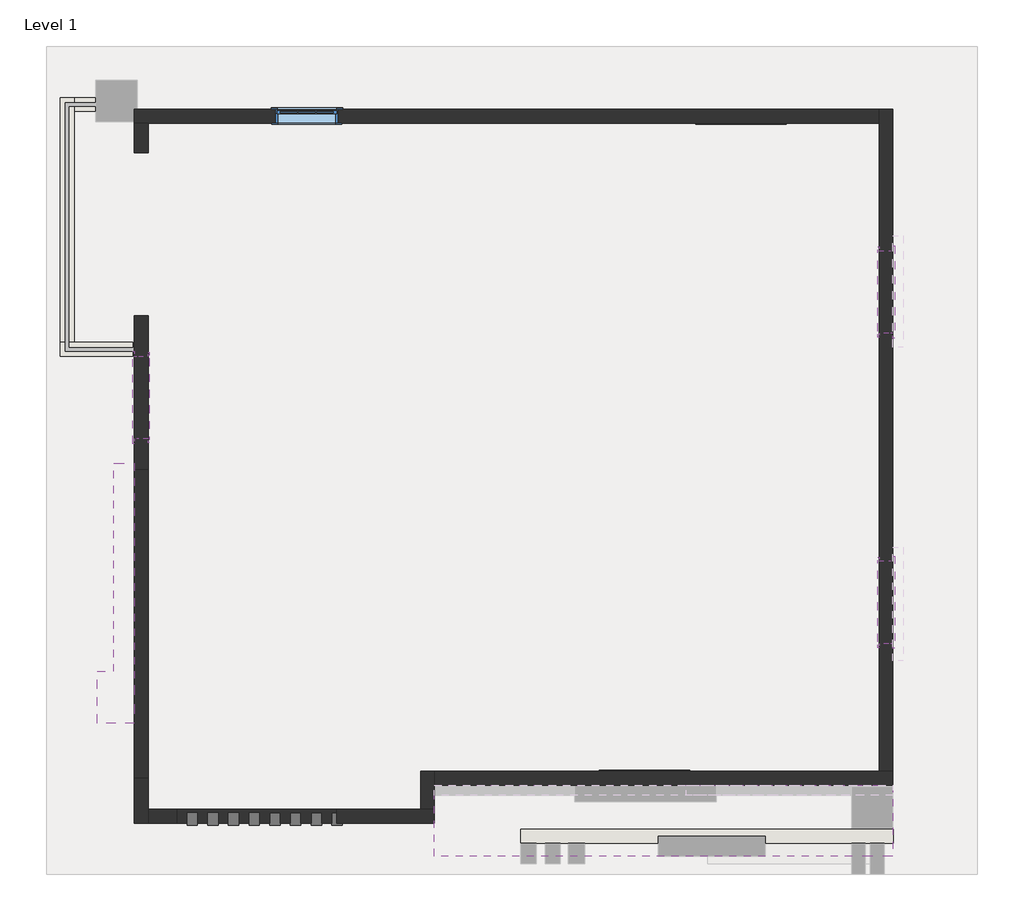
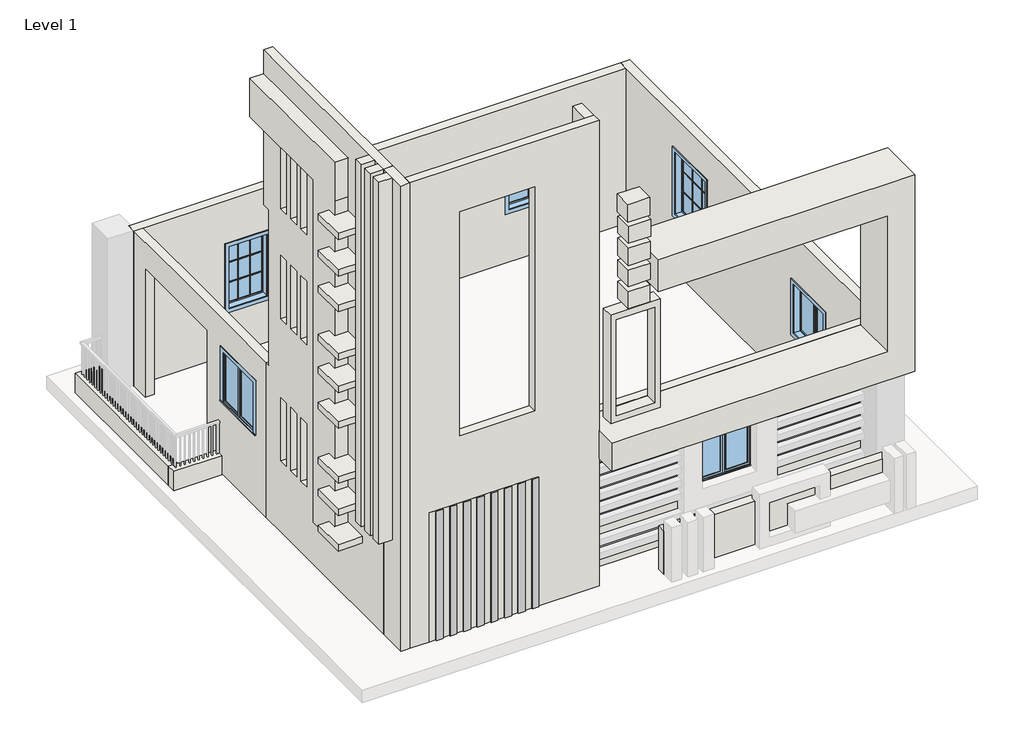
# One storey, part 1 of 2: 15 walls, 8 proxies, 6 windows.
"""IFC4 building model written with IfcOpenShell, lengths in millimetres."""

from ifc_helpers import new_model, si_unit, origin, origin_with_axes, place, context, project, spatial, polyline, outline, extrude, faceted_brep, transform, mapped, element, save
from components import walls_1_walls_1_66469eba, walls_2_walls_2_6b9d7f67, window_58e1470a, window_26ecbd3e, window_0862ab64

model = new_model("IFC4")

# Units and contexts
model_context = context("Model", 3, world=origin())
ifc_project = project(units=[si_unit("LENGTHUNIT", "METRE", prefix="MILLI")], contexts=[model_context])

# Site, building, storey
site = spatial("IfcSite", under=ifc_project)
building = spatial("IfcBuilding", under=site)
storey = spatial("IfcBuildingStorey", under=building, Name="Level 1", Elevation=0.0)

# Proxies
placement = place(None, origin())
element("IfcBuildingElementProxy", 1, Name="Reveal", ObjectType="Reveal", at=placement, inside=storey, context=model_context, shape_type="SweptSolid", body=[
    extrude(outline(polyline([(-11010.4950134, -2653.806099), (-11010.4950134, -2470.926099), (-10858.0950134, -2470.926099), (-10858.0950134, -2653.806099), (-11010.4950134, -2653.806099)])), origin_with_axes(), (0.0, 0.0, 1.0), 3049.7998229),
])
element("IfcBuildingElementProxy", 2, Name="Reveal", ObjectType="Reveal", at=placement, inside=storey, context=model_context, shape_type="SweptSolid", body=[
    extrude(outline(polyline([(-10705.6950134, -2653.806099), (-10705.6950134, -2470.926099), (-10553.2950134, -2470.926099), (-10553.2950134, -2653.806099), (-10705.6950134, -2653.806099)])), origin_with_axes(), (0.0, 0.0, 1.0), 3049.7998229),
])
element("IfcBuildingElementProxy", 3, Name="Reveal", ObjectType="Reveal", at=placement, inside=storey, context=model_context, shape_type="SweptSolid", body=[
    extrude(outline(polyline([(-10400.8950134, -2653.806099), (-10400.8950134, -2470.926099), (-10248.4950134, -2470.926099), (-10248.4950134, -2653.806099), (-10400.8950134, -2653.806099)])), origin_with_axes(), (0.0, 0.0, 1.0), 3049.7998229),
])
element("IfcBuildingElementProxy", 4, Name="Reveal", ObjectType="Reveal", at=placement, inside=storey, context=model_context, shape_type="SweptSolid", body=[
    extrude(outline(polyline([(-10096.0950134, -2653.806099), (-10096.0950134, -2470.926099), (-9943.6950134, -2470.926099), (-9943.6950134, -2653.806099), (-10096.0950134, -2653.806099)])), origin_with_axes(), (0.0, 0.0, 1.0), 3049.7998229),
])
element("IfcBuildingElementProxy", 5, Name="Reveal", ObjectType="Reveal", at=placement, inside=storey, context=model_context, shape_type="SweptSolid", body=[
    extrude(outline(polyline([(-9791.2950134, -2653.806099), (-9791.2950134, -2470.926099), (-9638.8950134, -2470.926099), (-9638.8950134, -2653.806099), (-9791.2950134, -2653.806099)])), origin_with_axes(), (0.0, 0.0, 1.0), 3049.7998229),
])
element("IfcBuildingElementProxy", 6, Name="Reveal", ObjectType="Reveal", at=placement, inside=storey, context=model_context, shape_type="SweptSolid", body=[
    extrude(outline(polyline([(-9486.4950134, -2653.806099), (-9486.4950134, -2470.926099), (-9334.0950134, -2470.926099), (-9334.0950134, -2653.806099), (-9486.4950134, -2653.806099)])), origin_with_axes(), (0.0, 0.0, 1.0), 3049.7998229),
])
element("IfcBuildingElementProxy", 7, Name="Reveal", ObjectType="Reveal", at=placement, inside=storey, context=model_context, shape_type="SweptSolid", body=[
    extrude(outline(polyline([(-9181.6950134, -2653.806099), (-9181.6950134, -2470.926099), (-9029.2950134, -2470.926099), (-9029.2950134, -2653.806099), (-9181.6950134, -2653.806099)])), origin_with_axes(), (0.0, 0.0, 1.0), 3049.7998229),
])
element("IfcBuildingElementProxy", 8, Name="Reveal", ObjectType="Reveal", at=placement, inside=storey, context=model_context, shape_type="SweptSolid", body=[
    extrude(outline(polyline([(-8876.8950134, -2653.806099), (-8876.8950134, -2470.926099), (-8724.4950134, -2470.926099), (-8724.4950134, -2653.806099), (-8876.8950134, -2653.806099)])), origin_with_axes(), (0.0, 0.0, 1.0), 3049.7998229),
])

# Walls
element("IfcWall", 9, ObjectType="Generic - 8\"", at=placement, inside=storey, context=model_context, shape_type="Brep", body=[
    faceted_brep([(-11786.2932708, 7689.073901, 0.0), (-11583.0932708, 7689.073901, 0.0), (-813.4932708, 7689.073901, 0.0), (-813.4932708, 7689.073901, 3657.6), (-11583.0932708, 7689.073901, 3657.6), (-11786.2932708, 7689.073901, 3657.6), (-8789.0932708, 7689.073901, 2590.7953104), (-8789.0932708, 7689.073901, 1066.7953104), (-9703.4932708, 7689.073901, 1066.7953104), (-9703.4932708, 7689.073901, 2590.7953104), (-2235.8932708, 7689.073901, 2428.7388642), (-2235.8932708, 7689.073901, 1209.5388642), (-3455.0932708, 7689.073901, 1209.5388642), (-3455.0932708, 7689.073901, 2428.7388642), (-11786.2932708, 7892.273901, 0.0), (-11786.2932708, 7892.273901, 3657.6), (-11742.7083357, 7892.273901, 3657.6), (-813.4932708, 7892.273901, 3657.6), (-813.4932708, 7892.273901, 0.0), (-11742.7083357, 7892.273901, 0.0), (-8789.0932708, 7892.273901, 2590.7953104), (-9703.4932708, 7892.273901, 2590.7953104), (-9703.4932708, 7892.273901, 1066.7953104), (-8789.0932708, 7892.273901, 1066.7953104), (-2235.8932708, 7892.273901, 2428.7388642), (-3455.0932708, 7892.273901, 2428.7388642), (-3455.0932708, 7892.273901, 1209.5388642), (-2235.8932708, 7892.273901, 1209.5388642), (-11786.2932708, 7709.3483652, 0.0), (-11786.2932708, 7709.3483652, 3657.6)], [[[0, 1, 2, 3, 4, 5], [6, 7, 8, 9], [10, 11, 12, 13]], [[14, 15, 16, 17, 18, 19], [20, 21, 22, 23], [24, 25, 26, 27]], [[2, 1, 0, 28, 14, 19, 18]], [[5, 4, 3, 17, 16, 15, 29]], [[0, 5, 29, 15, 14, 28]], [[3, 2, 18, 17]], [[7, 6, 20, 23]], [[8, 7, 23, 22]], [[9, 8, 22, 21]], [[6, 9, 21, 20]], [[11, 10, 24, 27]], [[12, 11, 27, 26]], [[13, 12, 26, 25]], [[10, 13, 25, 24]]]),
])
element("IfcWall", 10, ObjectType="Generic - 8\"", at=placement, inside=storey, context=model_context, shape_type="Brep", body=[
    faceted_brep([(-11583.0932708, 2578.5483652, 3657.6), (-11583.0932708, 2578.5483652, 0.0), (-11583.0932708, 4851.2528272, 0.0), (-11583.0932708, 4851.2528272, 3042.8682475), (-11583.0932708, 7251.0434239, 3042.8682475), (-11583.0932708, 7251.0434239, 0.0), (-11583.0932708, 7689.073901, 0.0), (-11583.0932708, 7689.073901, 3657.6), (-11583.0932708, 5905.4772304, 3657.6), (-11583.0932708, 4533.8772304, 3657.6), (-11583.0932708, 4254.9483652, 2926.4797977), (-11583.0932708, 4254.9483652, 1707.2797977), (-11583.0932708, 3035.7483652, 1707.2797977), (-11583.0932708, 3035.7483652, 2926.4797977), (-11786.2932708, 2578.5483652, 0.0), (-11786.2932708, 2578.5483652, 3657.6), (-11786.2932708, 4533.8772304, 3657.6), (-11786.2932708, 5905.4772304, 3657.6), (-11786.2932708, 7689.073901, 3657.6), (-11786.2932708, 7689.073901, 0.0), (-11786.2932708, 7251.0434239, 0.0), (-11786.2932708, 7251.0434239, 3042.8682475), (-11786.2932708, 4851.2528272, 3042.8682475), (-11786.2932708, 4851.2528272, 0.0), (-11786.2932708, 4254.9483652, 2926.4797977), (-11786.2932708, 3035.7483652, 2926.4797977), (-11786.2932708, 3035.7483652, 1707.2797977), (-11786.2932708, 4254.9483652, 1707.2797977)], [[[0, 1, 2, 3, 4, 5, 6, 7, 8, 9], [10, 11, 12, 13]], [[14, 15, 16, 17, 18, 19, 20, 21, 22, 23], [24, 25, 26, 27]], [[7, 6, 19, 18]], [[11, 10, 24, 27]], [[12, 11, 27, 26]], [[13, 12, 26, 25]], [[10, 13, 25, 24]], [[0, 9, 8, 7, 18, 17, 16, 15]], [[0, 15, 14, 1]], [[2, 1, 14, 23]], [[3, 2, 23, 22]], [[4, 3, 22, 21]], [[5, 4, 21, 20]], [[6, 5, 20, 19]]]),
])
element("IfcWall", 11, ObjectType="Generic - 8\"", at=placement, inside=storey, context=model_context, shape_type="Brep", body=[
    faceted_brep([(-610.2932708, -1861.326099, 0.0), (-813.4932708, -1861.326099, 0.0), (-7366.6932708, -1861.326099, 0.0), (-7366.6932708, -1861.326099, 3657.6), (-813.4932708, -1861.326099, 3657.6), (-610.2932708, -1861.326099, 3657.6), (-4877.4932708, -1861.326099, 2439.58165), (-4877.4932708, -1861.326099, 1220.38165), (-3658.2932708, -1861.326099, 1220.38165), (-3658.2932708, -1861.326099, 2439.58165), (-610.2932708, -2064.526099, 0.0), (-610.2932708, -2064.526099, 3657.6), (-7366.6932708, -2064.526099, 3657.6), (-7366.6932708, -2064.526099, 0.0), (-4877.4932708, -2064.526099, 2439.58165), (-3658.2932708, -2064.526099, 2439.58165), (-3658.2932708, -2064.526099, 1220.38165), (-4877.4932708, -2064.526099, 1220.38165)], [[[0, 1, 2, 3, 4, 5], [6, 7, 8, 9]], [[10, 11, 12, 13], [14, 15, 16, 17]], [[2, 1, 0, 10, 13]], [[5, 4, 3, 12, 11]], [[0, 5, 11, 10]], [[3, 2, 13, 12]], [[7, 6, 14, 17]], [[8, 7, 17, 16]], [[9, 8, 16, 15]], [[6, 9, 15, 14]]]),
])
element("IfcWall", 12, ObjectType="Generic - 8\"", at=placement, inside=storey, context=model_context, shape_type="Brep", body=[
    faceted_brep([(-813.4932708, 7892.273901, 0.0), (-813.4932708, 7689.073901, 0.0), (-813.4932708, -1861.326099, 0.0), (-813.4932708, -1861.326099, 3657.6), (-813.4932708, 7689.073901, 3657.6), (-813.4932708, 7892.273901, 3657.6), (-813.4932708, 4590.273901, 2873.0721634), (-813.4932708, 4590.273901, 1349.0721634), (-813.4932708, 5809.473901, 1349.0721634), (-813.4932708, 5809.473901, 2873.0721634), (-813.4932708, 18.273901, 2533.8575763), (-813.4932708, 18.273901, 1314.6575763), (-813.4932708, 1237.473901, 1314.6575763), (-813.4932708, 1237.473901, 2533.8575763), (-610.2932708, 7892.273901, 0.0), (-610.2932708, 7892.273901, 3657.6), (-610.2932708, -1861.326099, 3657.6), (-610.2932708, -1861.326099, 0.0), (-610.2932708, 4590.273901, 2873.0721634), (-610.2932708, 5809.473901, 2873.0721634), (-610.2932708, 5809.473901, 1349.0721634), (-610.2932708, 4590.273901, 1349.0721634), (-610.2932708, 18.273901, 2533.8575763), (-610.2932708, 1237.473901, 2533.8575763), (-610.2932708, 1237.473901, 1314.6575763), (-610.2932708, 18.273901, 1314.6575763)], [[[0, 1, 2, 3, 4, 5], [6, 7, 8, 9], [10, 11, 12, 13]], [[14, 15, 16, 17], [18, 19, 20, 21], [22, 23, 24, 25]], [[2, 1, 0, 14, 17]], [[5, 4, 3, 16, 15]], [[0, 5, 15, 14]], [[3, 2, 17, 16]], [[7, 6, 18, 21]], [[8, 7, 21, 20]], [[9, 8, 20, 19]], [[6, 9, 19, 18]], [[11, 10, 22, 25]], [[12, 11, 25, 24]], [[13, 12, 24, 23]], [[10, 13, 23, 22]]]),
])
element("IfcWall", 13, ObjectType="Generic - 8\"", at=placement, inside=storey, context=model_context, shape_type="Brep", body=[
    faceted_brep([(-11786.2932708, 2578.5483652, 0.0), (-11786.2932708, -1962.926099, 0.0), (-11786.2932708, -1962.926099, 10972.8), (-11786.2932708, 2680.1483652, 10972.8), (-11786.2932708, 2680.1483652, 7315.2), (-11786.2932708, 2603.9483652, 7315.2), (-11786.2932708, 2476.9483652, 7315.2), (-11786.2932708, 2476.9483652, 3657.6), (-11786.2932708, 2578.5483652, 3657.6), (-11786.2932708, 1806.5522738, 9112.4526323), (-11786.2932708, 1806.5522738, 7620.0), (-11786.2932708, 2020.5114253, 7620.0), (-11786.2932708, 2020.5114253, 9112.4526323), (-11786.2932708, 1401.155987, 9112.4526323), (-11786.2932708, 1401.155987, 7620.0), (-11786.2932708, 1637.6371543, 7620.0), (-11786.2932708, 1637.6371543, 9112.4526323), (-11786.2932708, 1009.8986921, 9112.4526323), (-11786.2932708, 1009.8986921, 7620.0), (-11786.2932708, 1235.1188515, 7620.0), (-11786.2932708, 1235.1188515, 9112.4526323), (-11786.2932708, 1806.5522738, 6521.6526323), (-11786.2932708, 1806.5522738, 5029.2), (-11786.2932708, 2020.5114253, 5029.2), (-11786.2932708, 2020.5114253, 6521.6526323), (-11786.2932708, 1401.155987, 6521.6526323), (-11786.2932708, 1401.155987, 5029.2), (-11786.2932708, 1637.6371543, 5029.2), (-11786.2932708, 1637.6371543, 6521.6526323), (-11786.2932708, 1009.8986921, 6521.6526323), (-11786.2932708, 1009.8986921, 5029.2), (-11786.2932708, 1235.1188515, 5029.2), (-11786.2932708, 1235.1188515, 6521.6526323), (-11786.2932708, 1806.5522738, 3168.8526323), (-11786.2932708, 1806.5522738, 1676.4), (-11786.2932708, 2020.5114253, 1676.4), (-11786.2932708, 2020.5114253, 3168.8526323), (-11786.2932708, 1401.155987, 3168.8526323), (-11786.2932708, 1401.155987, 1676.4), (-11786.2932708, 1637.6371543, 1676.4), (-11786.2932708, 1637.6371543, 3168.8526323), (-11786.2932708, 1009.8986921, 3168.8526323), (-11786.2932708, 1009.8986921, 1676.4), (-11786.2932708, 1235.1188515, 1676.4), (-11786.2932708, 1235.1188515, 3168.8526323), (-11583.0932708, 2578.5483652, 0.0), (-11583.0932708, 2578.5483652, 3657.6), (-11583.0932708, 2476.9483652, 3657.6), (-11583.0932708, 2476.9483652, 7315.2), (-11583.0932708, 2680.1483652, 7315.2), (-11583.0932708, 2680.1483652, 10972.8), (-11583.0932708, 2476.9483652, 10972.8), (-11583.0932708, -1962.926099, 10972.8), (-11583.0932708, -1962.926099, 0.0), (-11583.0932708, 1806.5522738, 9112.4526323), (-11583.0932708, 2020.5114253, 9112.4526323), (-11583.0932708, 2020.5114253, 7620.0), (-11583.0932708, 1806.5522738, 7620.0), (-11583.0932708, 1401.155987, 9112.4526323), (-11583.0932708, 1637.6371543, 9112.4526323), (-11583.0932708, 1637.6371543, 7620.0), (-11583.0932708, 1401.155987, 7620.0), (-11583.0932708, 1009.8986921, 9112.4526323), (-11583.0932708, 1235.1188515, 9112.4526323), (-11583.0932708, 1235.1188515, 7620.0), (-11583.0932708, 1009.8986921, 7620.0), (-11583.0932708, 1806.5522738, 6521.6526323), (-11583.0932708, 2020.5114253, 6521.6526323), (-11583.0932708, 2020.5114253, 5029.2), (-11583.0932708, 1806.5522738, 5029.2), (-11583.0932708, 1401.155987, 6521.6526323), (-11583.0932708, 1637.6371543, 6521.6526323), (-11583.0932708, 1637.6371543, 5029.2), (-11583.0932708, 1401.155987, 5029.2), (-11583.0932708, 1009.8986921, 6521.6526323), (-11583.0932708, 1235.1188515, 6521.6526323), (-11583.0932708, 1235.1188515, 5029.2), (-11583.0932708, 1009.8986921, 5029.2), (-11583.0932708, 1806.5522738, 3168.8526323), (-11583.0932708, 2020.5114253, 3168.8526323), (-11583.0932708, 2020.5114253, 1676.4), (-11583.0932708, 1806.5522738, 1676.4), (-11583.0932708, 1401.155987, 3168.8526323), (-11583.0932708, 1637.6371543, 3168.8526323), (-11583.0932708, 1637.6371543, 1676.4), (-11583.0932708, 1401.155987, 1676.4), (-11583.0932708, 1009.8986921, 3168.8526323), (-11583.0932708, 1235.1188515, 3168.8526323), (-11583.0932708, 1235.1188515, 1676.4), (-11583.0932708, 1009.8986921, 1676.4)], [[[0, 1, 2, 3, 4, 5, 6, 7, 8], [9, 10, 11, 12], [13, 14, 15, 16], [17, 18, 19, 20], [21, 22, 23, 24], [25, 26, 27, 28], [29, 30, 31, 32], [33, 34, 35, 36], [37, 38, 39, 40], [41, 42, 43, 44]], [[45, 46, 47, 48, 49, 50, 51, 52, 53], [54, 55, 56, 57], [58, 59, 60, 61], [62, 63, 64, 65], [66, 67, 68, 69], [70, 71, 72, 73], [74, 75, 76, 77], [78, 79, 80, 81], [82, 83, 84, 85], [86, 87, 88, 89]], [[3, 2, 52, 51, 50]], [[6, 48, 47, 7]], [[1, 0, 45, 53]], [[2, 1, 53, 52]], [[0, 8, 46, 45]], [[7, 47, 46, 8]], [[4, 49, 48, 6, 5]], [[10, 9, 54, 57]], [[11, 10, 57, 56]], [[12, 11, 56, 55]], [[9, 12, 55, 54]], [[14, 13, 58, 61]], [[15, 14, 61, 60]], [[16, 15, 60, 59]], [[13, 16, 59, 58]], [[18, 17, 62, 65]], [[19, 18, 65, 64]], [[20, 19, 64, 63]], [[17, 20, 63, 62]], [[22, 21, 66, 69]], [[23, 22, 69, 68]], [[24, 23, 68, 67]], [[21, 24, 67, 66]], [[26, 25, 70, 73]], [[27, 26, 73, 72]], [[28, 27, 72, 71]], [[25, 28, 71, 70]], [[30, 29, 74, 77]], [[31, 30, 77, 76]], [[32, 31, 76, 75]], [[29, 32, 75, 74]], [[34, 33, 78, 81]], [[35, 34, 81, 80]], [[36, 35, 80, 79]], [[33, 36, 79, 78]], [[38, 37, 82, 85]], [[39, 38, 85, 84]], [[40, 39, 84, 83]], [[37, 40, 83, 82]], [[42, 41, 86, 89]], [[43, 42, 89, 88]], [[44, 43, 88, 87]], [[41, 44, 87, 86]], [[3, 50, 49, 4]]]),
])
element("IfcWall", 14, ObjectType="Generic - 8\"", at=placement, inside=storey, context=model_context, shape_type="Brep", body=[
    faceted_brep([(-7366.6932708, -2420.126099, 10972.8), (-7366.6932708, -2420.126099, 0.0), (-7569.8932708, -2420.126099, 0.0), (-8801.0344883, -2420.126099, 0.0), (-8801.0344883, -2420.126099, 3049.7998229), (-11162.8950134, -2420.126099, 3049.7998229), (-11162.8950134, -2420.126099, 0.0), (-11583.0932708, -2420.126099, 0.0), (-11583.0932708, -2420.126099, 10972.8), (-7569.8932708, -2420.126099, 10972.8), (-8801.0344883, -2420.126099, 9908.1845939), (-10477.4344883, -2420.126099, 9908.1845939), (-10477.4344883, -2420.126099, 4624.9845939), (-8801.0344883, -2420.126099, 4624.9845939), (-7366.6932708, -2623.326099, 0.0), (-7366.6932708, -2623.326099, 10972.8), (-11583.0932708, -2623.326099, 10972.8), (-11583.0932708, -2623.326099, 0.0), (-11162.8950134, -2623.326099, 0.0), (-11162.8950134, -2623.326099, 3049.7998229), (-11010.4950134, -2623.326099, 3049.7998229), (-10858.0950134, -2623.326099, 3049.7998229), (-10705.6950134, -2623.326099, 3049.7998229), (-10553.2950134, -2623.326099, 3049.7998229), (-10400.8950134, -2623.326099, 3049.7998229), (-10248.4950134, -2623.326099, 3049.7998229), (-10096.0950134, -2623.326099, 3049.7998229), (-9943.6950134, -2623.326099, 3049.7998229), (-9791.2950134, -2623.326099, 3049.7998229), (-9638.8950134, -2623.326099, 3049.7998229), (-9486.4950134, -2623.326099, 3049.7998229), (-9334.0950134, -2623.326099, 3049.7998229), (-9181.6950134, -2623.326099, 3049.7998229), (-9029.2950134, -2623.326099, 3049.7998229), (-8876.8950134, -2623.326099, 3049.7998229), (-8801.0344883, -2623.326099, 3049.7998229), (-8801.0344883, -2623.326099, 0.0), (-8801.0344883, -2623.326099, 9908.1845939), (-8801.0344883, -2623.326099, 4624.9845939), (-10477.4344883, -2623.326099, 4624.9845939), (-10477.4344883, -2623.326099, 9908.1845939), (-8801.0344883, -2470.926099, 0.0), (-8801.0344883, -2470.926099, 3049.7998229)], [[[0, 1, 2, 3, 4, 5, 6, 7, 8, 9], [10, 11, 12, 13]], [[14, 15, 16, 17, 18, 19, 20, 21, 22, 23, 24, 25, 26, 27, 28, 29, 30, 31, 32, 33, 34, 35, 36], [37, 38, 39, 40]], [[8, 7, 17, 16]], [[0, 9, 8, 16, 15]], [[11, 10, 37, 40]], [[12, 11, 40, 39]], [[13, 12, 39, 38]], [[10, 13, 38, 37]], [[0, 15, 14, 1]], [[3, 2, 1, 14, 36, 41]], [[4, 3, 41, 36, 35, 42]], [[5, 4, 42, 35, 34, 33, 32, 31, 30, 29, 28, 27, 26, 25, 24, 23, 22, 21, 20, 19]], [[6, 5, 19, 18]], [[7, 6, 18, 17]]]),
])
element("IfcWall", 15, ObjectType="Generic - 8\"", at=placement, inside=storey, context=model_context, shape_type="Brep", body=[
    faceted_brep([(-11786.2932708, -1962.926099, 0.0), (-11786.2932708, -2623.326099, 0.0), (-11786.2932708, -2623.326099, 10972.8), (-11786.2932708, -1962.926099, 10972.8), (-11583.0932708, -1962.926099, 0.0), (-11583.0932708, -1962.926099, 10972.8), (-11583.0932708, -2420.126099, 10972.8), (-11583.0932708, -2623.326099, 10972.8), (-11583.0932708, -2623.326099, 0.0), (-11583.0932708, -2420.126099, 0.0)], [[[0, 1, 2, 3]], [[4, 5, 6, 7, 8, 9]], [[1, 0, 4, 9, 8]], [[0, 3, 5, 4]], [[2, 1, 8, 7]], [[3, 2, 7, 6, 5]]]),
])
element("IfcWall", 16, ObjectType="Generic - 8\"", at=placement, inside=storey, context=model_context, shape_type="Brep", body=[
    faceted_brep([(-7366.6932708, -2420.126099, 10972.8), (-7366.6932708, -2420.126099, 0.0), (-7366.6932708, -2064.526099, 0.0), (-7366.6932708, -1861.326099, 0.0), (-7366.6932708, -1861.326099, 3657.6), (-7366.6932708, -1861.326099, 7315.2), (-7366.6932708, -1962.926099, 7315.2), (-7366.6932708, -1962.926099, 10972.8), (-7569.8932708, -2420.126099, 0.0), (-7569.8932708, -2420.126099, 10972.8), (-7569.8932708, -1962.926099, 10972.8), (-7569.8932708, -1962.926099, 7315.2), (-7569.8932708, -1861.326099, 7315.2), (-7569.8932708, -1861.326099, 0.0)], [[[0, 1, 2, 3, 4, 5, 6, 7]], [[8, 9, 10, 11, 12, 13]], [[3, 2, 1, 8, 13]], [[0, 7, 10, 9]], [[7, 6, 11, 10]], [[11, 6, 5, 12]], [[5, 4, 3, 13, 12]], [[0, 9, 8, 1]]]),
])
element("IfcWall", 17, ObjectType="Generic - 8\"", at=placement, inside=storey, context=model_context, shape_type="Brep", body=[
    faceted_brep([(-11811.6932708, 4458.1483652, 0.0), (-12675.2932708, 4458.1483652, 0.0), (-12878.4932708, 4458.1483652, 0.0), (-12878.4932708, 4458.1483652, 457.2), (-12675.2932708, 4458.1483652, 457.2), (-11811.6932708, 4458.1483652, 457.2), (-11811.6932708, 4254.9483652, 0.0), (-11811.6932708, 4254.9483652, 457.2), (-12878.4932708, 4254.9483652, 457.2), (-12878.4932708, 4254.9483652, 0.0)], [[[0, 1, 2, 3, 4, 5]], [[6, 7, 8, 9]], [[2, 1, 0, 6, 9]], [[5, 4, 3, 8, 7]], [[0, 5, 7, 6]], [[3, 2, 9, 8]]]),
])
element("IfcWall", 18, ObjectType="Generic - 8\"", at=placement, inside=storey, context=model_context, shape_type="Brep", body=[
    faceted_brep([(-12675.2932708, 4458.1483652, 0.0), (-12675.2932708, 7861.7483652, 0.0), (-12675.2932708, 8064.9483652, 0.0), (-12675.2932708, 8064.9483652, 457.2), (-12675.2932708, 7861.7483652, 457.2), (-12675.2932708, 4458.1483652, 457.2), (-12878.4932708, 4458.1483652, 0.0), (-12878.4932708, 4458.1483652, 457.2), (-12878.4932708, 8064.9483652, 457.2), (-12878.4932708, 8064.9483652, 0.0)], [[[0, 1, 2, 3, 4, 5]], [[6, 7, 8, 9]], [[2, 1, 0, 6, 9]], [[5, 4, 3, 8, 7]], [[0, 5, 7, 6]], [[3, 2, 9, 8]]]),
])
element("IfcWall", 19, ObjectType="Generic - 8\"", at=placement, inside=storey, context=model_context, shape_type="SweptSolid", body=[
    extrude(outline(polyline([(-12352.3083357, 7861.7483652), (-12675.2932708, 7861.7483652), (-12675.2932708, 8064.9483652), (-12352.3083357, 8064.9483652), (-12352.3083357, 7861.7483652)])), origin_with_axes(), (0.0, 0.0, 1.0), 457.2),
])
element("IfcWall", 20, ObjectType="Generic - 8\"", at=placement, inside=storey, context=model_context, shape_type="SweptSolid", body=[
    extrude(outline(polyline([(-607.3940307, -2919.855266), (-6093.7940307, -2919.855266), (-6093.7940307, -2716.655266), (-607.3940307, -2716.655266), (-607.3940307, -2919.855266)])), origin_with_axes(), (0.0, 0.0, 1.0), 1025.2624899),
])
element("IfcWall", 21, ObjectType="Generic - 8\"", at=placement, inside=storey, context=model_context, shape_type="SweptSolid", body=[
    extrude(outline(polyline([(-11162.8950134, -2420.126099), (-8801.0344883, -2420.126099), (-8801.0344883, -2470.926099), (-8876.8950134, -2470.926099), (-8876.8950134, -2623.326099), (-9029.2950134, -2623.326099), (-9029.2950134, -2470.926099), (-9181.6950134, -2470.926099), (-9181.6950134, -2623.326099), (-9334.0950134, -2623.326099), (-9334.0950134, -2470.926099), (-9486.4950134, -2470.926099), (-9486.4950134, -2623.326099), (-9638.8950134, -2623.326099), (-9638.8950134, -2470.926099), (-9791.2950134, -2470.926099), (-9791.2950134, -2623.326099), (-9943.6950134, -2623.326099), (-9943.6950134, -2470.926099), (-10096.0950134, -2470.926099), (-10096.0950134, -2623.326099), (-10248.4950134, -2623.326099), (-10248.4950134, -2470.926099), (-10400.8950134, -2470.926099), (-10400.8950134, -2623.326099), (-10553.2950134, -2623.326099), (-10553.2950134, -2470.926099), (-10705.6950134, -2470.926099), (-10705.6950134, -2623.326099), (-10858.0950134, -2623.326099), (-10858.0950134, -2470.926099), (-11010.4950134, -2470.926099), (-11010.4950134, -2623.326099), (-11162.8950134, -2623.326099), (-11162.8950134, -2420.126099)])), origin_with_axes(), (0.0, 0.0, 1.0), 3049.7998229),
])
walls_1_walls_1_shape = walls_1_walls_1_66469eba(model_context)
element("IfcWall", 22, ObjectType="Walls 1 : Walls 1", at=placement, inside=storey, context=model_context, shape_type="MappedRepresentation", body=[
    mapped(walls_1_walls_1_shape, transform((0.0, 0.0, 0.0), x_axis=(1.0, 0.0, 0.0), y_axis=(0.0, 1.0, 0.0), z_axis=(0.0, 0.0, 1.0))),
])
walls_2_walls_2_shape = walls_2_walls_2_6b9d7f67(model_context)
element("IfcWall", 23, ObjectType="Walls 2 : Walls 2", at=placement, inside=storey, context=model_context, shape_type="MappedRepresentation", body=[
    mapped(walls_2_walls_2_shape, transform((0.0, 0.0, 0.0), x_axis=(1.0, 0.0, 0.0), y_axis=(0.0, 1.0, 0.0), z_axis=(0.0, 0.0, 1.0))),
])

# Windows
window_shape = window_58e1470a(model_context)
element("IfcWindow", 24, ObjectType="Casement 3x3 with Trim : 36\" x 60\"", at=placement, inside=storey, context=model_context, shape_type="MappedRepresentation", body=[
    mapped(window_shape, transform((-9246.2932708, 7790.673901, 457.1953104), x_axis=(1.0, 0.0, 0.0), y_axis=(0.0, 1.0, 0.0), z_axis=(0.0, 0.0, 1.0))),
])
window_2_shape = window_26ecbd3e(model_context)
element("IfcWindow", 25, ObjectType="Casement 3x3 with Trim : 48\" x 60\"", at=placement, inside=storey, context=model_context, shape_type="MappedRepresentation", body=[
    mapped(window_2_shape, transform((-711.8932708, 5199.873901, 434.6721634), x_axis=(0.0, -1.0, 0.0), y_axis=(1.0, 0.0, 0.0), z_axis=(0.0, 0.0, 1.0))),
])
window_3_shape = window_0862ab64(model_context)
element("IfcWindow", 26, ObjectType="Casement Dbl with Trim.0001 : 48\" x 48\"", at=placement, inside=storey, context=model_context, shape_type="MappedRepresentation", body=[
    mapped(window_3_shape, transform((-11665.6432708, 3645.3483652, 792.8797977), x_axis=(0.0, 1.0, 0.0), y_axis=(-1.0, 0.0, 0.0), z_axis=(0.0, 0.0, 1.0))),
])
element("IfcWindow", 27, ObjectType="Casement Dbl with Trim.0001 : 48\" x 48\"", at=placement, inside=storey, context=model_context, shape_type="MappedRepresentation", body=[
    mapped(window_3_shape, transform((-4267.8932708, -1943.876099, 305.98165), x_axis=(-1.0, 0.0, 0.0), y_axis=(0.0, -1.0, 0.0), z_axis=(0.0, 0.0, 1.0))),
])
element("IfcWindow", 28, ObjectType="Casement Dbl with Trim.0001 : 48\" x 48\"", at=placement, inside=storey, context=model_context, shape_type="MappedRepresentation", body=[
    mapped(window_3_shape, transform((-730.9432708, 627.873901, 400.2575763), x_axis=(0.0, -1.0, 0.0), y_axis=(1.0, 0.0, 0.0), z_axis=(0.0, 0.0, 1.0))),
])
element("IfcWindow", 29, ObjectType="Casement Dbl with Trim.0001 : 48\" x 48\"", at=placement, inside=storey, context=model_context, shape_type="MappedRepresentation", body=[
    mapped(window_3_shape, transform((-2845.4932708, 7771.623901, 295.1388642), x_axis=(1.0, 0.0, 0.0), y_axis=(0.0, 1.0, 0.0), z_axis=(0.0, 0.0, 1.0))),
])

save(model, "model.ifc")

# Revit data of these elements
# Type "Generic - 8\""
#   Assembly Code = "B2010"
#   Layers, outside or top first: 0' - 8" no material (function 1)
# Type "Casement 3x3 with Trim : 36\" x 60\""
#   Type Mark = "14"
#   Construction Type Id = "GSP4R"
#   Assembly Code = "B2020100"
#   Analytic Construction = "1/8 in Pilkington single glazing"
#   Visual Light Transmittance = 0.9
#   Solar Heat Gain Coefficient = 0.78
#   Heat Transfer Coefficient (U) = 0.6496 BTU/(h·ft²·°F)
#   Height = 5' - 0"
#   Default Sill Height = 2' - 0"
#   Trim Projection - Ext. = 0' - 0 1/2"
#   Trim Projection - Int. = 0' - 0 3/4"
#   Trim Width - Exterior = 0' - 3 1/2"
#   Trim Width - Interior = 0' - 3 1/2"
#   Width = 3' - 0"
#   Window Inset = 0' - 0 3/4"
#   Define Thermal Properties by = 1
#   Glass Pane Material = Glass
#   Sash Material = Sash
#   Trim Exterior Material = Trim
#   Trim Interior Material = Trim
#   Wall Closure = (empty or 0)
# Type "Casement 3x3 with Trim : 48\" x 60\""
#   Type Mark = "13"
#   Construction Type Id = "GSP4R"
#   Assembly Code = "B2020100"
#   Analytic Construction = "1/8 in Pilkington single glazing"
#   Visual Light Transmittance = 0.9
#   Solar Heat Gain Coefficient = 0.78
#   Heat Transfer Coefficient (U) = 0.6496 BTU/(h·ft²·°F)
#   Height = 5' - 0"
#   Default Sill Height = 3' - 0"
#   Trim Projection - Ext. = 0' - 0 1/2"
#   Trim Projection - Int. = 0' - 0 3/4"
#   Trim Width - Exterior = 0' - 3 1/2"
#   Trim Width - Interior = 0' - 3 1/2"
#   Width = 4' - 0"
#   Window Inset = 0' - 0 3/4"
#   Define Thermal Properties by = 1
#   Glass Pane Material = Glass
#   Sash Material = Sash
#   Trim Exterior Material = Trim
#   Trim Interior Material = Trim
#   Wall Closure = (empty or 0)
# Type "Casement Dbl with Trim.0001 : 48\" x 48\""
#   Type Mark = "10"
#   Construction Type Id = "GSP4R"
#   Assembly Code = "B2020100"
#   Analytic Construction = "1/8 in Pilkington single glazing"
#   Visual Light Transmittance = 0.9
#   Solar Heat Gain Coefficient = 0.78
#   Heat Transfer Coefficient (U) = 0.6496 BTU/(h·ft²·°F)
#   Height = 4' - 0"
#   Default Sill Height = 3' - 0"
#   Trim Projection - Ext. = 0' - 0 1/2"
#   Trim Projection - Int. = 0' - 0 3/4"
#   Trim Width - Exterior = 0' - 3 1/2"
#   Trim Width - Interior = 0' - 3 1/2"
#   Width = 4' - 0"
#   Window Inset = 0' - 0 3/4"
#   Define Thermal Properties by = 1
#   Glass Pane Material = Glass
#   Sash Material = Sash
#   Trim Exterior Material = Trim
#   Trim Interior Material = Trim
#   Wall Closure = (empty or 0)
# Elements 9, 10, 11, 12 (IfcWall, "Generic - 8\"")
#   Top Offset = 0' - 0"
#   Base Offset = 0' - 0"
#   Unconnected Height = 12' - 0"
#   wall height = 12' - 0"
#   Phase Created = New Construction
#   Base Constraint = Level 1
#   Materials on its faces: "Default Wall"
# Element 13 (IfcWall, "Generic - 8\"")
#   Top Offset = 0' - 0"
#   Base Offset = 0' - 0"
#   Unconnected Height = 41' - 8.41068"
#   wall height = 41' - 8.41068"
#   Phase Created = New Construction
#   Base Constraint = Level 1
#   Materials on its faces: "Default Wall"
# Element 14 (IfcWall, "Generic - 8\"")
#   Top Offset = 0' - 0"
#   Base Offset = 0' - 0"
#   Unconnected Height = 42' - 1.36366"
#   wall height = 42' - 1.36366"
#   Phase Created = New Construction
#   Base Constraint = Level 1
#   Materials on its faces: "Default Wall"
# Element 15 (IfcWall, "Generic - 8\"")
#   Top Offset = 0' - 0"
#   Base Offset = 0' - 0"
#   Unconnected Height = 42' - 3.06013"
#   wall height = 42' - 3.06013"
#   Phase Created = New Construction
#   Base Constraint = Level 1
#   Materials on its faces: "Default Wall"
# Element 16 (IfcWall, "Generic - 8\"")
#   Top Offset = 0' - 0"
#   Base Offset = 0' - 0"
#   Unconnected Height = 42' - 2.80738"
#   wall height = 42' - 2.80738"
#   Phase Created = New Construction
#   Base Constraint = Level 1
#   Materials on its faces: "Default Wall"
# Elements 17, 18, 19 (IfcWall, "Generic - 8\"")
#   Top Offset = -10' - 6"
#   Base Offset = 0' - 0"
#   wall height = 1' - 6"
#   Phase Created = New Construction
#   Base Constraint = Level 1
#   Top Constraint = Level 2
#   Materials on its faces: "Default Wall"
# Element 20 (IfcWall, "Generic - 8\"")
#   Top Offset = 0' - 0"
#   Base Offset = 0' - 0"
#   Unconnected Height = 3' - 4.36466"
#   wall height = 3' - 4.36466"
#   Phase Created = New Construction
#   Base Constraint = Level 1
#   Materials on its faces: "Default Wall"
# Element 21 (IfcWall, "Generic - 8\"")
#   Top Offset = 0' - 0"
#   Base Offset = 0' - 0"
#   Unconnected Height = 10' - 0.07086"
#   wall height = 10' - 0.07086"
#   Phase Created = New Construction
#   Base Constraint = Level 1
#   Materials on its faces: "Default Wall"
# Element 22 (IfcWall, "Walls 1 : Walls 1")
#   Phase Created = New Construction
#   Materials on its faces: "Default Wall"
# Element 23 (IfcWall, "Walls 2 : Walls 2")
#   Phase Created = New Construction
#   Materials on its faces: "Default Wall"
# Element 24 (IfcWindow, "Casement 3x3 with Trim : 36\" x 60\"")
#   Mark = "9"
#   Phase Created = New Construction
#   Materials on its faces: "Sash", "Glass", "Trim"
# Element 25 (IfcWindow, "Casement 3x3 with Trim : 48\" x 60\"")
#   Mark = "5"
#   Phase Created = New Construction
#   Materials on its faces: "Sash", "Glass", "Trim"
# Element 26 (IfcWindow, "Casement Dbl with Trim.0001 : 48\" x 48\"")
#   Mark = "1"
#   Phase Created = New Construction
#   Materials on its faces: "Sash", "Trim", "Glass"
# Element 27 (IfcWindow, "Casement Dbl with Trim.0001 : 48\" x 48\"")
#   Mark = "3"
#   Phase Created = New Construction
#   Materials on its faces: "Sash", "Trim", "Glass"
# Element 28 (IfcWindow, "Casement Dbl with Trim.0001 : 48\" x 48\"")
#   Mark = "6"
#   Phase Created = New Construction
#   Materials on its faces: "Sash", "Trim", "Glass"
# Element 29 (IfcWindow, "Casement Dbl with Trim.0001 : 48\" x 48\"")
#   Mark = "10"
#   Phase Created = New Construction
#   Materials on its faces: "Sash", "Trim", "Glass"
# Materials
#   "Glass": class "Glass", colour RGB 0 128 192, transparency 0.75, Description = "Soda Lime Glass", Cost = 0
#   "Sash": class "Wood", colour RGB 224 178 126, transparency 0
#   "Trim": class "Wood", colour RGB 224 178 126, transparency 0
#   "Default Wall": colour RGB 128 128 128, transparency 0
